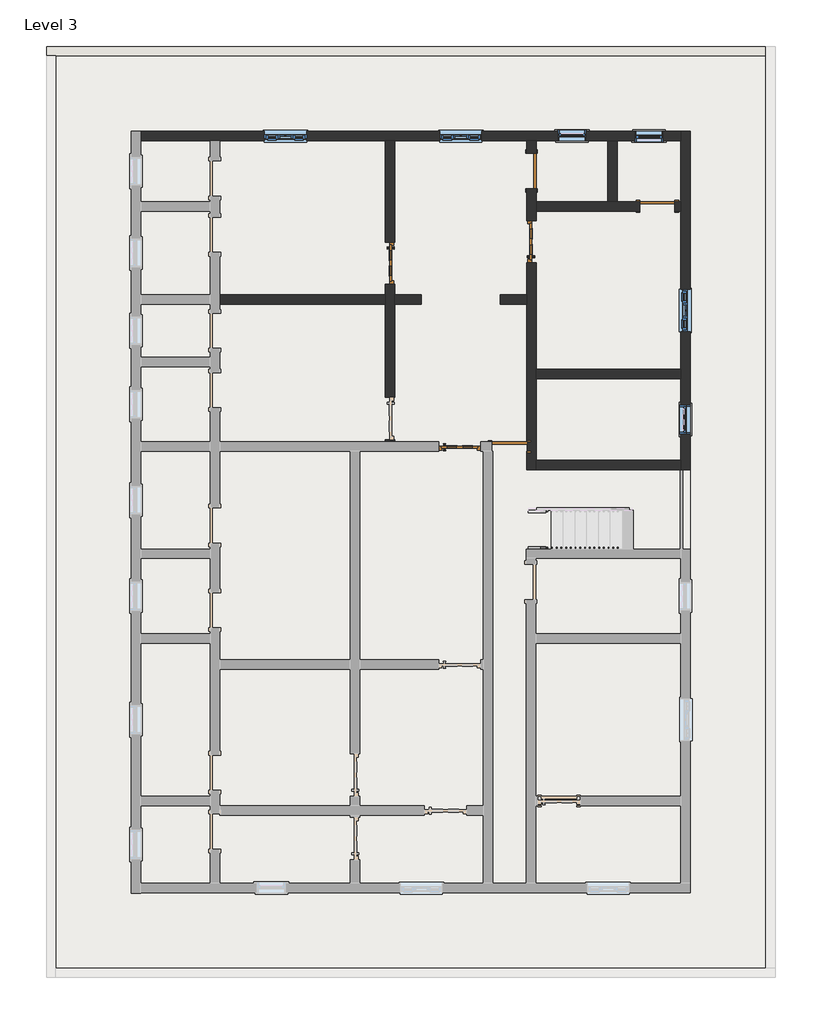
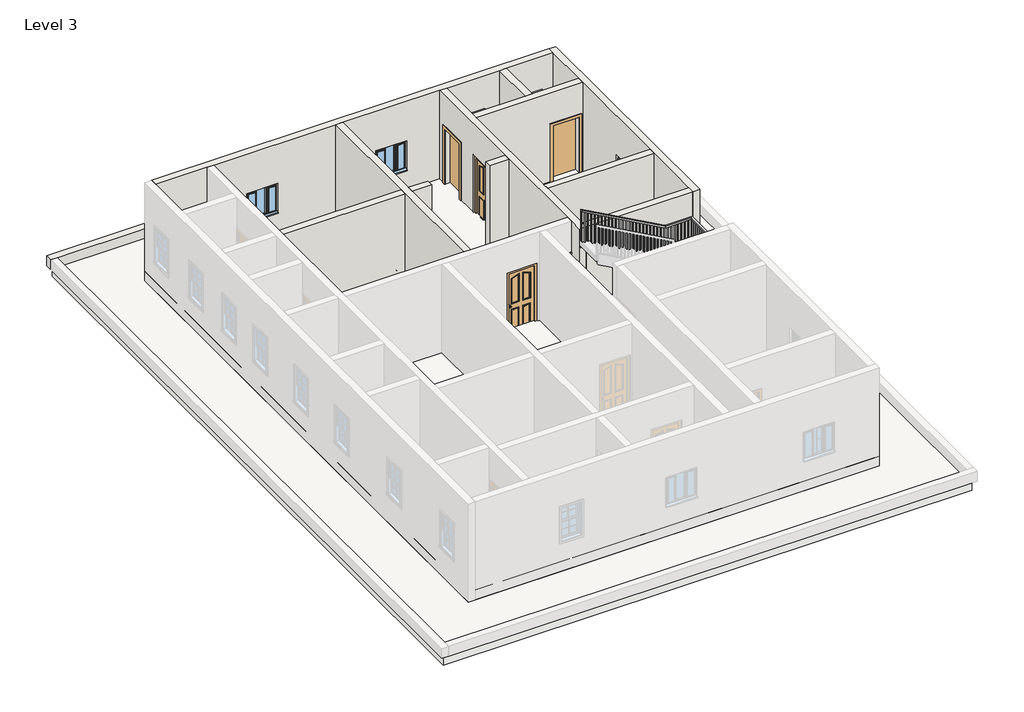
# One storey, part 2 of 3: 11 walls, 6 doors, 6 windows, 2 slabs, 1 railing, 1 roof.
# Revit data of these elements (continued)
# Type "Windows_Tpl_w-Glazing_Cross-Bars : 910x910mm" (continued)
#   Cavity Closer Depth = 0' - 3.34646"
#   Vis - Glazing Bars = yes
#   Vis - Cavity Closers = yes
#   Define Thermal Properties by = 1
#   Material Trim = Window Frame
#   Material Glazing Bars = Window Frame
#   Material Glass = Glass
#   Material Frame = Window Frame
#   Wall Closure = (empty or 0)
# Elements 1, 2, 3 (IfcDoor, "Doors_ExtSgl_12 : 910x2110mm")
#   Phase Created = New Construction
#   Materials on its faces: "Door - Panel", "Door - Handle", "Door - Frame/Mullion", "Door - Glazing"
# Elements 4, 5, 6 (IfcDoor, "Single-Flush : 30\" x 80\"")
#   Phase Created = New Construction
#   Materials on its faces: "Door - Frame", "Door - Panel"
# Element 7 (IfcRailing, "Handrail - Rectangular")
#   Phase Created = New Construction
# Element 8 (IfcRoof, "Generic - 12\"")
#   built-in parameter 1001705 = 21 (stored number, unit not read)
#   built-in parameter 1001710 = 33615
#   Phase Created = New Construction
#   Materials on its faces: "Default Roof"
# Elements 9, 10 (IfcSlab, "Generic - 12\"")
#   Height Offset From Level = 0' - 0"
#   Phase Created = New Construction
#   Materials on its faces: "Default Floor"
# Elements 11, 12, 13, 14, 15, 16, 17, 18 (IfcWall, "4.5\"")
#   Top Offset = 0' - 0"
#   Base Offset = 0' - 0"
#   wall height = 10' - 0"
#   Phase Created = New Construction
#   Base Constraint = Level 3
#   Top Constraint = Level 4
#   Materials on its faces: "Default Wall"
# Element 19 (IfcWall, "4.5\"")
#   Top Offset = 0' - 0"
#   Base Offset = 0' - 0"
#   Unconnected Height = 1' - 0"
#   wall height = 1' - 0"
#   Phase Created = New Construction
#   Base Constraint = Level 3
#   Materials on its faces: "Default Wall"
# Elements 20, 21 (IfcWall, "Generic - 9\"")
#   Top Offset = 0' - 0"
#   Base Offset = 0' - 0"
#   wall height = 10' - 0"
#   Phase Created = New Construction
#   Base Constraint = Level 3
#   Top Constraint = Level 4
#   Materials on its faces: "Default Wall", "Tile, Porcelain, 4in"
# Element 22 (IfcWindow, "Window-Double-Hung : 24\" x 42\"")
#   Mark = "52"
#   Window Inset = 0' - 0"
#   Interior Wall Closure = 0' - 1 1/2"
#   Frame Extension = 0' - 1 1/4"
#   Exterior Wall Closure = 0' - 0 1/2"
#   Interior Trim Visibility = yes
#   Indicator Visibility = yes
#   Exterior Trim Visibility = yes
#   Phase Created = New Construction
#   Materials on its faces: "Wood - Stained", "Glass", "Clad - White"
# Element 23 (IfcWindow, "Window-Double-Hung : 24\" x 42\"")
#   Mark = "53"
#   Window Inset = 0' - 0"
#   Interior Wall Closure = 0' - 1 1/2"
#   Frame Extension = 0' - 1 1/4"
#   Exterior Wall Closure = 0' - 0 1/2"
#   Interior Trim Visibility = yes
#   Indicator Visibility = yes
#   Exterior Trim Visibility = yes
#   Phase Created = New Construction
#   Materials on its faces: "Wood - Stained", "Glass", "Clad - White"
# Element 24 (IfcWindow, "Window-Double-Hung : 24\" x 42\"")
#   Mark = "54"
#   Window Inset = 0' - 0"
#   Interior Wall Closure = 0' - 1 1/2"
#   Frame Extension = 0' - 1 1/4"
#   Exterior Wall Closure = 0' - 0 1/2"
#   Interior Trim Visibility = yes
#   Indicator Visibility = yes
#   Exterior Trim Visibility = yes
#   Phase Created = New Construction
#   Materials on its faces: "Wood - Stained", "Glass", "Clad - White"
# Element 25 (IfcWindow, "Windows_Tpl_w-Glazing_Cross-Bars : 910x910mm")
#   Mark = "40"
#   Phase Created = New Construction
#   Materials on its faces: "Window Frame", "Glass"
# Element 26 (IfcWindow, "Windows_Tpl_w-Glazing_Cross-Bars : 910x910mm")
#   Mark = "41"
#   Phase Created = New Construction
#   Materials on its faces: "Window Frame", "Glass"
# Element 27 (IfcWindow, "Windows_Tpl_w-Glazing_Cross-Bars : 910x910mm")
#   Mark = "55"
#   Phase Created = New Construction
#   Materials on its faces: "Window Frame", "Glass"
# Materials
#   "Door - Glazing": colour RGB 0 0 255, transparency 0.75
#   "Door - Panel": class "Wood", colour RGB 210 159 95, transparency 0, Cost = 0
#   "Door - Frame/Mullion": class "Wood", colour RGB 212 179 113, transparency 0
#   "Door - Handle": colour RGB 246 240 166, transparency 0
#   "Door - Frame": colour RGB 118 70 51, transparency 0, Cost = 0
#   "Wood - Stained": class "Wood", colour RGB 224 178 126, transparency 0, Cost = 0
#   "Clad - White": class "Wood", colour RGB 242 242 238, transparency 0, Cost = 0
#   "Glass": class "Glass", colour RGB 0 128 192, transparency 0.75, Description = "Soda Lime Glass", Cost = 0
#   "Window Frame": colour RGB 249 249 249, transparency 0
#   "Default Roof": colour RGB 88 101 114, transparency 0, Cost = 0
#   "Default Floor": colour RGB 128 128 128, transparency 0, Cost = 0
#   "Default Wall": colour RGB 128 128 128, transparency 0, Cost = 0
#   "Tile, Porcelain, 4in": class "Generic", colour RGB 89 87 158, transparency 0, Description = "Porcelain tile, 4\", white", Cost = 0
